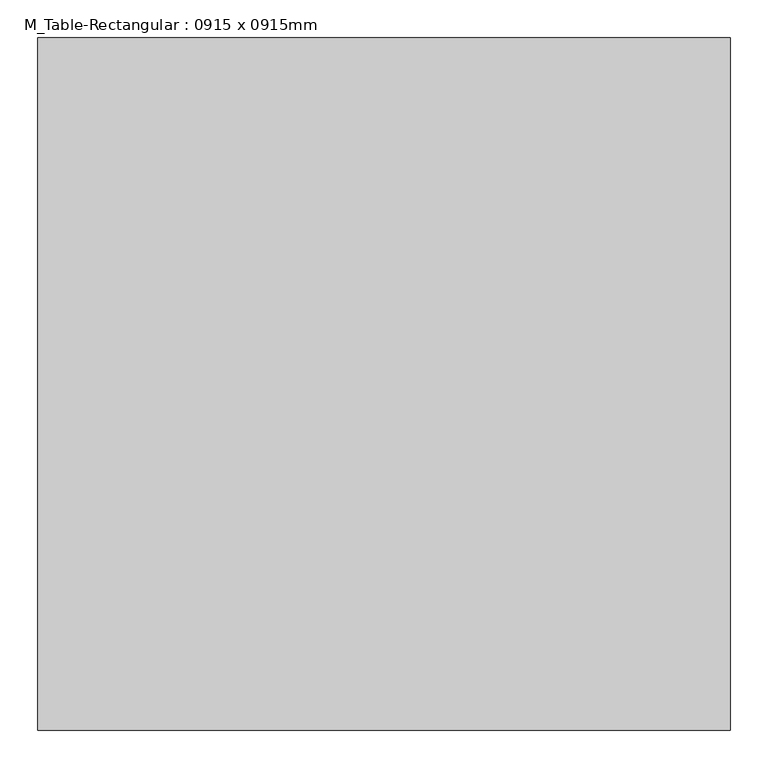
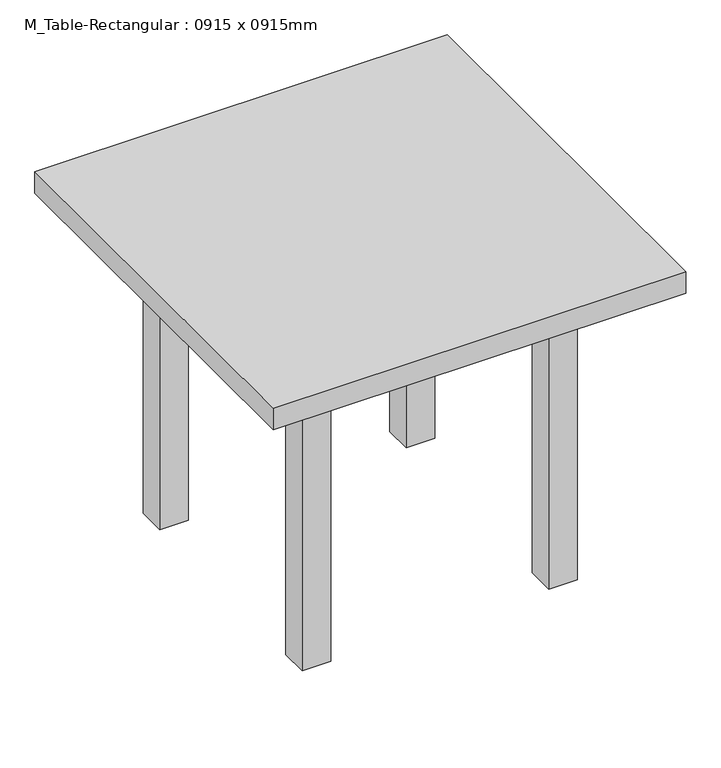
"""IFC4 building model written with IfcOpenShell, lengths in millimetres: furniture geometry, M_Table-Rectangular : 0915 x 0915mm."""

from ifc_helpers import new_model, si_unit, frame, origin, origin_with_axes, place, context, project, spatial, polyline, outline, extrude, source, transform, mapped, element, save


def m_table_rectangular_0915_x_0915mm_8578315f(model_context):
    return source(origin(), model_context, "Body", "SweptSolid", [
        extrude(outline(polyline([(241.6, 267.0), (241.6, 241.6), (-241.6, 241.6), (-241.6, 267.0), (241.6, 267.0)])), frame((0.0, 0.0, 609.6), z_axis=(0.0, 0.0, 1.0), x_axis=(1.0, 0.0, 0.0)), (0.0, 0.0, 1.0), 101.6),
        extrude(outline(polyline([(241.6, -267.0), (-241.6, -267.0), (-241.6, -241.6), (241.6, -241.6), (241.6, -267.0)])), frame((0.0, 0.0, 609.6), z_axis=(0.0, 0.0, 1.0), x_axis=(1.0, 0.0, 0.0)), (0.0, 0.0, 1.0), 101.6),
        extrude(outline(polyline([(-254.3, -241.6), (-279.7, -241.6), (-279.7, 241.6), (-254.3, 241.6), (-254.3, -241.6)])), frame((0.0, 0.0, 609.6), z_axis=(0.0, 0.0, 1.0), x_axis=(1.0, 0.0, 0.0)), (0.0, 0.0, 1.0), 101.6),
        extrude(outline(polyline([(254.3, -241.6), (254.3, 241.6), (279.7, 241.6), (279.7, -241.6), (254.3, -241.6)])), frame((0.0, 0.0, 609.6), z_axis=(0.0, 0.0, 1.0), x_axis=(1.0, 0.0, 0.0)), (0.0, 0.0, 1.0), 101.6),
        extrude(outline(polyline([(457.5, 457.5), (457.5, -457.5), (-457.5, -457.5), (-457.5, 457.5), (457.5, 457.5)])), frame((0.0, 0.0, 711.2), z_axis=(0.0, 0.0, 1.0), x_axis=(1.0, 0.0, 0.0)), (0.0, 0.0, 1.0), 50.8),
        extrude(outline(polyline([(-241.6, 305.1), (-241.6, 241.6), (-305.1, 241.6), (-305.1, 305.1), (-241.6, 305.1)])), origin_with_axes(), (0.0, 0.0, 1.0), 711.2),
        extrude(outline(polyline([(241.6, 305.1), (305.1, 305.1), (305.1, 241.6), (241.6, 241.6), (241.6, 305.1)])), origin_with_axes(), (0.0, 0.0, 1.0), 711.2),
        extrude(outline(polyline([(-241.6, -305.1), (-305.1, -305.1), (-305.1, -241.6), (-241.6, -241.6), (-241.6, -305.1)])), origin_with_axes(), (0.0, 0.0, 1.0), 711.2),
        extrude(outline(polyline([(241.6, -305.1), (241.6, -241.6), (305.1, -241.6), (305.1, -305.1), (241.6, -305.1)])), origin_with_axes(), (0.0, 0.0, 1.0), 711.2),
    ])


if __name__ == "__main__":
    model = new_model("IFC4")
    model_context = context("Model", 3, world=origin())
    ifc_project = project(units=[si_unit("LENGTHUNIT", "METRE", prefix="MILLI")], contexts=[model_context])
    site = spatial("IfcSite", under=ifc_project)
    building = spatial("IfcBuilding", under=site)
    placement = place(None, origin())
    m_table_rectangular_0915_x_0915mm_shape = m_table_rectangular_0915_x_0915mm_8578315f(model_context)
    element("IfcFurniture", 1, ObjectType="M_Table-Rectangular : 0915 x 0915mm", at=placement, inside=building, context=model_context, shape_type="MappedRepresentation", body=[
        mapped(m_table_rectangular_0915_x_0915mm_shape, transform((0.0, 0.0, 0.0), x_axis=(1.0, 0.0, 0.0), y_axis=(0.0, 1.0, 0.0), z_axis=(0.0, 0.0, 1.0))),
    ])
    save(model, "model.ifc")

# Revit data of these elements
# Type "M_Table-Rectangular : 0915 x 0915mm"
#   Height = 2' - 6"
#   Length = 3' - 0.02362"
#   Width = 3' - 0.02362"
#   Base Material = Birch
#   Top Material = Birch
#   Default Elevation = 0
# Element 1 (IfcFurniture, "M_Table-Rectangular : 0915 x 0915mm")
#   Materials on its faces: "Birch"
# Materials
#   "Birch": class "Wood", colour RGB 224 178 126, transparency 0, Description = "Betula Alleghaniensis", Cost = 0
